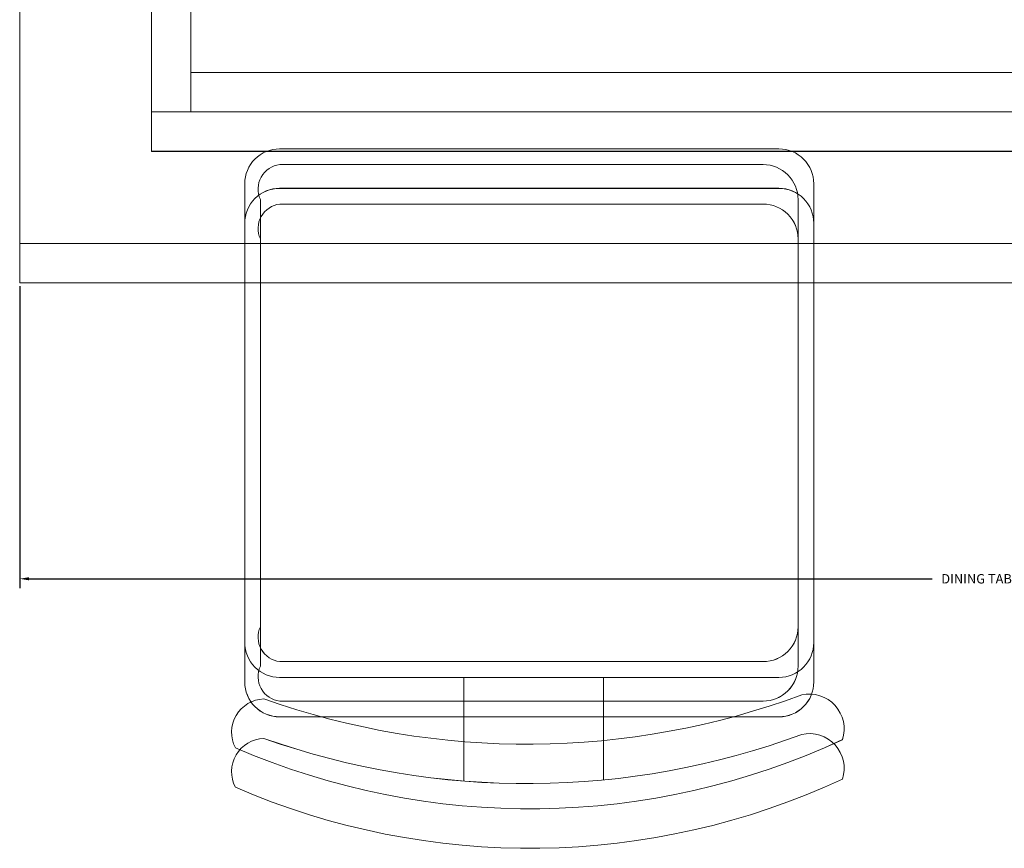
# Model space of a CAD drawing. Units: inches. Extents: x 1885 to 2748, y 783 to 2421.
# Tile 23 of 117: x 2348.64 to 2367.48, y 1245.44 to 1261.31. Entities that reach past the tile are written whole.
import ezdxf

# ---------------------------------------------------------------- set-up
doc = ezdxf.new("R2010")
doc.units = ezdxf.units.IN
doc.layers.add('A-ANNO-DIMS', color=2, linetype='Continuous', lineweight=18)
doc.layers.add('A-FURN', color=8, linetype='Continuous', lineweight=13)
doc.styles.get("Standard").update_dxf_attribs({"font": 'arial.ttf'})
doc.dimstyles.get("Standard").update_dxf_attribs({"dimtxt": 0.18, "dimasz": 0.18, "dimexe": 0.18, "dimexo": 0.0625, "dimgap": 0.09, "dimtad": 0, "dimtih": 1, "dimtoh": 1, "dimdec": 4, "dimzin": 0, "dimdsep": 46, "dimtxsty": 'Standard', "dimcen": 0.09, "dimadec": 0, "dimazin": 0, "dimtfac": 1, "dimtdec": 4, "dimtofl": 0, "dimtmove": 0, "dimatfit": 3, "dimfxl": 1, "dimtolj": 1, "dimtzin": 0, "dimarcsym": 0})

# ---------------------------------------------------------------- blocks, each defined once
blk = doc.blocks.new('TABLE-DINING-RECT')
for points in [[(-0.004, 23.421), (37.776, 23.421), (37.776, 0.754), (-0.004, 0.754)], [(-0.004, 23.421), (37.776, 23.421), (37.776, 0.753), (-0.004, 0.753)], [(-0.004, 22.666), (37.776, 22.666), (37.776, -0.002), (-0.004, -0.002)], [(-0.004, 22.665), (37.776, 22.665), (37.776, -0.002), (-0.004, -0.002)], [(2.515, 20.903), (35.257, 20.903), (35.257, 3.272), (2.515, 3.272)], [(2.515, 20.902), (35.257, 20.902), (35.257, 3.272), (2.515, 3.272)], [(2.515, 20.147), (35.257, 20.147), (35.257, 2.517), (2.515, 2.517)], [(2.515, 20.147), (35.257, 20.147), (35.257, 2.516), (2.515, 2.516)], [(3.27, 20.147), (34.501, 20.147), (34.501, 4.028), (3.27, 4.028)], [(3.27, 20.147), (34.501, 20.147), (34.501, 4.027), (3.27, 4.027)], [(3.27, 19.391), (34.501, 19.391), (34.501, 3.272), (3.27, 3.272)], [(3.27, 19.391), (34.501, 19.391), (34.501, 3.272), (3.27, 3.272)]]:
    blk.add_lwpolyline(points, close=True)
blk = doc.blocks.new('*D35')
at = {"layer": 'A-ANNO-DIMS', "color": 0, "lineweight": -2, "transparency": 16777216}
for p, q in [((2348.636, 1256.205), (2348.636, 1250.421)), ((2386.416, 1256.205), (2386.416, 1250.421)), ((2348.816, 1250.601), (2366.094, 1250.601)), ((2386.236, 1250.601), (2368.958, 1250.601))]:
    blk.add_line(p, q, dxfattribs=at)
at = {"layer": 'A-ANNO-DIMS', "color": 0, "transparency": 16777216}
for points in [[(2348.816, 1250.631), (2348.816, 1250.571), (2348.636, 1250.601)], [(2386.236, 1250.631), (2386.236, 1250.571), (2386.416, 1250.601)]]:
    blk.add_solid(points, dxfattribs=at)
at = {"layer": 'Defpoints', "color": 0, "transparency": 16777216}
for p in [(2348.636, 1256.268), (2386.416, 1256.268), (2386.416, 1250.601)]:
    blk.add_point(p, dxfattribs=at)
at = {"layer": 'A-ANNO-DIMS', "color": 0, "transparency": 16777216, "insert": (2367.526, 1250.601), "char_height": 0.18, "attachment_point": 5}
blk.add_mtext('\\A1;DINING TABLE 38 TYP.', dxfattribs=at)

msp = doc.modelspace()

# ---------------------------------------------------------------- linework, layer by layer
at = {"layer": 'A-FURN'}
for points in [[(2363.163, 1248.713), (2353.61, 1248.713, -0.414214), (2352.941, 1249.381), (2352.941, 1258.165, -0.414214), (2353.61, 1258.833), (2363.163, 1258.833, -0.414214), (2363.831, 1258.165), (2363.831, 1249.381, -0.414214), (2363.163, 1248.713)], [(2363.163, 1248.713), (2353.61, 1248.713, -0.414214), (2352.941, 1249.381), (2352.941, 1258.165, -0.414214), (2353.61, 1258.833), (2363.163, 1258.833, -0.414214), (2363.831, 1258.165), (2363.831, 1249.381, -0.414214), (2363.163, 1248.713)], [(2363.163, 1247.958), (2353.61, 1247.958, -0.414214), (2352.941, 1248.626), (2352.941, 1257.41, -0.414214), (2353.61, 1258.078), (2363.163, 1258.078, -0.414214), (2363.831, 1257.41), (2363.831, 1248.626, -0.414214), (2363.163, 1247.958)], [(2363.163, 1247.957), (2353.61, 1247.957, -0.414214), (2352.941, 1248.625), (2352.941, 1257.409, -0.414214), (2353.61, 1258.077), (2363.163, 1258.077, -0.414214), (2363.831, 1257.409), (2363.831, 1248.625, -0.414214), (2363.163, 1247.957)], [(2359.807, 1248.713), (2359.807, 1247.505, 0.064759)], [(2359.807, 1248.713), (2359.807, 1247.505, 0.064759)], [(2363.599, 1248.378, -0.578392), (2364.379, 1247.521, -0.214524), (2352.763, 1247.365, -0.552014), (2353.309, 1248.3, 0.175809), (2363.599, 1248.378)], [(2363.599, 1248.378, -0.578392), (2364.379, 1247.52, -0.214524), (2352.763, 1247.365, -0.552014), (2353.309, 1248.3, 0.175809), (2363.599, 1248.378)], [(2359.807, 1247.958), (2359.807, 1246.749, 0.064759)], [(2359.807, 1247.957), (2359.807, 1246.749, 0.064759)], [(2363.599, 1247.622, -0.578392), (2364.379, 1246.765, -0.214524), (2352.763, 1246.609, -0.552014), (2353.309, 1247.545, 0.175809), (2363.599, 1247.622)], [(2363.599, 1247.622, -0.578392), (2364.379, 1246.765, -0.214524), (2352.763, 1246.609, -0.552014), (2353.309, 1247.544, 0.175809), (2363.599, 1247.622)]]:
    msp.add_lwpolyline(points, format="xyb", dxfattribs=at)
for points in [[(2353.614, 1249.014), (2362.862, 1249.014, 0.414214), (2363.53, 1249.683), (2363.53, 1257.864, 0.414214), (2362.862, 1258.532), (2353.614, 1258.532, 0.512069), (2353.242, 1257.864), (2353.242, 1249.683, 0.512069)], [(2353.614, 1249.014), (2362.862, 1249.014, 0.414214), (2363.53, 1249.682), (2363.53, 1257.864, 0.414214), (2362.862, 1258.532), (2353.614, 1258.532, 0.512069), (2353.242, 1257.864), (2353.242, 1249.682, 0.512069)], [(2353.614, 1248.259), (2362.862, 1248.259, 0.414214), (2363.53, 1248.927), (2363.53, 1257.108, 0.414214), (2362.862, 1257.777), (2353.614, 1257.777, 0.512069), (2353.242, 1257.108), (2353.242, 1248.927, 0.512069)], [(2353.614, 1248.258), (2362.862, 1248.258, 0.414214), (2363.53, 1248.927), (2363.53, 1257.108, 0.414214), (2362.862, 1257.776), (2353.614, 1257.776, 0.512069), (2353.242, 1257.108), (2353.242, 1248.927, 0.512069)]]:
    msp.add_lwpolyline(points, format="xyb", close=True, dxfattribs=at)
for points in [[(2357.133, 1247.483), (2357.133, 1248.713)], [(2357.133, 1247.483), (2357.133, 1248.713)], [(2357.133, 1246.727), (2357.133, 1247.958)], [(2357.133, 1246.727), (2357.133, 1247.957)]]:
    msp.add_lwpolyline(points, dxfattribs=at)

# ---------------------------------------------------------------- block references
msp.add_blockref('TABLE-DINING-RECT', (2348.64, 1256.27), dxfattribs=at)

# ---------------------------------------------------------------- dimensions: what is measured, and where the dimension line sits
at = {"layer": 'A-ANNO-DIMS'}
dim = msp.add_linear_dim(base=(2386.416, 1250.601), p1=(2348.636, 1256.268), p2=(2386.416, 1256.268), text='DINING TABLE <> TYP.', dimstyle='Standard', override={"dimdec": 0, "dimlfac": 1, "dimrnd": 0, "dimzin": 0, "dimdsep": 46, "dimlunit": 2}, dxfattribs=at)
dim.commit()
dim.dimension.update_dxf_attribs({"geometry": '*D35', "text_midpoint": (2367.526, 1250.601)})

doc.saveas('drawing.dxf')
